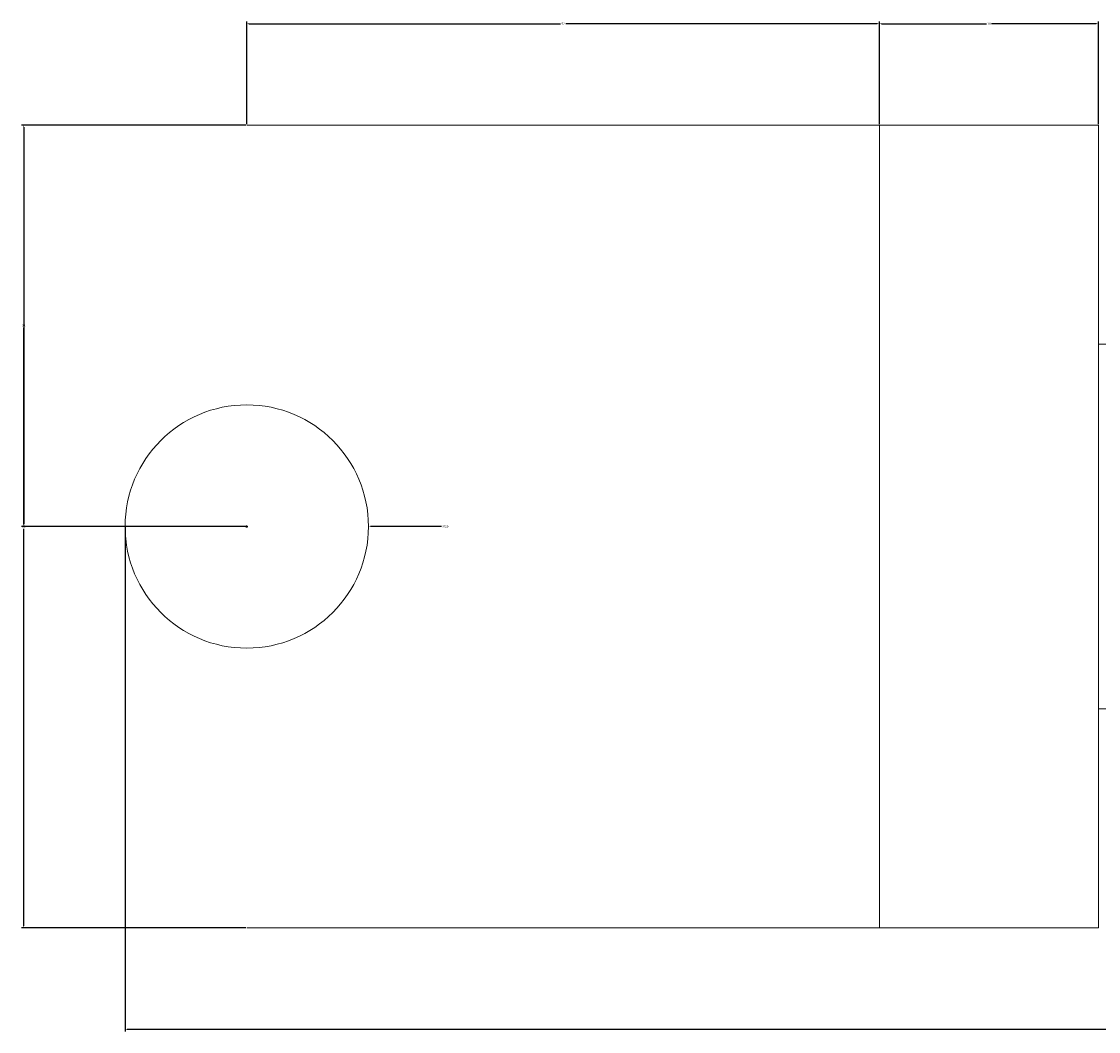
# Model space of a CAD drawing. Units: millimetres. Extents: x 2117 to 2298, y 1328 to 1411.
# Tile 1 of 3: x 2117 to 2205, y 1328 to 1411. Entities that reach past the tile are written whole.
import ezdxf

# ---------------------------------------------------------------- set-up
doc = ezdxf.new("R2010")
doc.units = ezdxf.units.MM
doc.layers.add('M-CONS', color=8, linetype='Continuous', lineweight=18)
doc.layers.add('M-DIMS', color=2, linetype='Continuous', lineweight=18)
doc.styles.get("Standard").update_dxf_attribs({"font": 'arial.ttf'})
doc.dimstyles.get("Standard").update_dxf_attribs({"dimtxt": 0.18, "dimasz": 0.18, "dimexe": 0.18, "dimexo": 0.0625, "dimgap": 0.09, "dimtad": 0, "dimtih": 1, "dimtoh": 1, "dimdec": 4, "dimzin": 0, "dimdsep": 46, "dimtxsty": 'Standard', "dimcen": 0.09, "dimadec": 0, "dimazin": 0, "dimtfac": 1, "dimtdec": 4, "dimtofl": 0, "dimtmove": 0, "dimatfit": 3, "dimfxl": 1, "dimtolj": 1, "dimtzin": 0, "dimarcsym": 0})

# ---------------------------------------------------------------- blocks, each defined once
blk = doc.blocks.new('*D3')
at = {"layer": 'Defpoints', "color": 0, "transparency": 16777216}
for p in [(2117.086, 1402.783), (2135.416, 1402.783), (2135.416, 1369.783)]:
    blk.add_point(p, dxfattribs=at)
at = {"layer": 'M-DIMS', "color": 0, "lineweight": -2, "transparency": 16777216}
for p, q in [((2135.354, 1402.783), (2116.906, 1402.783)), ((2117.086, 1402.603), (2117.086, 1386.465)), ((2117.086, 1369.963), (2117.086, 1386.101)), ((2135.354, 1369.783), (2116.906, 1369.783))]:
    blk.add_line(p, q, dxfattribs=at)
at = {"layer": 'M-DIMS', "color": 0, "transparency": 16777216}
for points in [[(2117.056, 1402.603), (2117.116, 1402.603), (2117.086, 1402.783)], [(2117.056, 1369.963), (2117.116, 1369.963), (2117.086, 1369.783)]]:
    blk.add_solid(points, dxfattribs=at)
at = {"layer": 'M-DIMS', "color": 0, "transparency": 16777216, "insert": (2117.086, 1386.283), "char_height": 0.18, "attachment_point": 5}
blk.add_mtext('\\A1;33', dxfattribs=at)
blk = doc.blocks.new('*D4')
at = {"layer": 'Defpoints', "color": 0, "transparency": 16777216}
for p in [(2117.086, 1402.783), (2135.416, 1402.783), (2135.416, 1336.783)]:
    blk.add_point(p, dxfattribs=at)
at = {"layer": 'M-DIMS', "color": 0, "lineweight": -2, "transparency": 16777216}
for p, q in [((2135.354, 1402.783), (2116.906, 1402.783)), ((2117.086, 1402.603), (2117.086, 1369.965)), ((2117.086, 1336.963), (2117.086, 1369.601)), ((2135.354, 1336.783), (2116.906, 1336.783))]:
    blk.add_line(p, q, dxfattribs=at)
at = {"layer": 'M-DIMS', "color": 0, "transparency": 16777216}
for points in [[(2117.056, 1402.603), (2117.116, 1402.603), (2117.086, 1402.783)], [(2117.056, 1336.963), (2117.116, 1336.963), (2117.086, 1336.783)]]:
    blk.add_solid(points, dxfattribs=at)
at = {"layer": 'M-DIMS', "color": 0, "transparency": 16777216, "insert": (2117.086, 1369.783), "char_height": 0.18, "attachment_point": 5}
blk.add_mtext('\\A1;66', dxfattribs=at)
blk = doc.blocks.new('*D5')
at = {"layer": 'Defpoints', "color": 0, "transparency": 16777216}
for p in [(2187.416, 1411.113), (2135.416, 1402.783), (2187.416, 1402.783)]:
    blk.add_point(p, dxfattribs=at)
at = {"layer": 'M-DIMS', "color": 0, "lineweight": -2, "transparency": 16777216}
for p, q in [((2135.416, 1402.845), (2135.416, 1411.293)), ((2135.596, 1411.113), (2161.198, 1411.113)), ((2187.236, 1411.113), (2161.634, 1411.113)), ((2187.416, 1402.845), (2187.416, 1411.293))]:
    blk.add_line(p, q, dxfattribs=at)
at = {"layer": 'M-DIMS', "color": 0, "transparency": 16777216}
for points in [[(2135.596, 1411.143), (2135.596, 1411.083), (2135.416, 1411.113)], [(2187.236, 1411.143), (2187.236, 1411.083), (2187.416, 1411.113)]]:
    blk.add_solid(points, dxfattribs=at)
at = {"layer": 'M-DIMS', "color": 0, "transparency": 16777216, "insert": (2161.416, 1411.113), "char_height": 0.18, "attachment_point": 5}
blk.add_mtext('\\A1;52', dxfattribs=at)
blk = doc.blocks.new('*D6')
at = {"layer": 'Defpoints', "color": 0, "transparency": 16777216}
for p in [(2205.416, 1411.113), (2187.416, 1402.783), (2205.416, 1402.783)]:
    blk.add_point(p, dxfattribs=at)
at = {"layer": 'M-DIMS', "color": 0, "lineweight": -2, "transparency": 16777216}
for p, q in [((2187.416, 1402.845), (2187.416, 1411.293)), ((2187.596, 1411.113), (2196.205, 1411.113)), ((2205.236, 1411.113), (2196.627, 1411.113)), ((2205.416, 1402.845), (2205.416, 1411.293))]:
    blk.add_line(p, q, dxfattribs=at)
at = {"layer": 'M-DIMS', "color": 0, "transparency": 16777216}
for points in [[(2187.596, 1411.143), (2187.596, 1411.083), (2187.416, 1411.113)], [(2205.236, 1411.143), (2205.236, 1411.083), (2205.416, 1411.113)]]:
    blk.add_solid(points, dxfattribs=at)
at = {"layer": 'M-DIMS', "color": 0, "transparency": 16777216, "insert": (2196.416, 1411.113), "char_height": 0.18, "attachment_point": 5}
blk.add_mtext('\\A1;18', dxfattribs=at)
blk = doc.blocks.new('*D12')
at = {"layer": 'Defpoints', "color": 0, "transparency": 16777216}
for p in [(2125.416, 1369.783), (2289.916, 1354.783), (2289.916, 1328.453)]:
    blk.add_point(p, dxfattribs=at)
at = {"layer": 'M-DIMS', "color": 0, "lineweight": -2, "transparency": 16777216}
for p, q in [((2125.416, 1369.72), (2125.416, 1328.273)), ((2289.916, 1354.72), (2289.916, 1328.273)), ((2125.596, 1328.453), (2207.28, 1328.453)), ((2289.736, 1328.453), (2208.052, 1328.453))]:
    blk.add_line(p, q, dxfattribs=at)
at = {"layer": 'M-DIMS', "color": 0, "transparency": 16777216}
for points in [[(2125.596, 1328.483), (2125.596, 1328.423), (2125.416, 1328.453)], [(2289.736, 1328.483), (2289.736, 1328.423), (2289.916, 1328.453)]]:
    blk.add_solid(points, dxfattribs=at)
at = {"layer": 'M-DIMS', "color": 0, "transparency": 16777216, "insert": (2207.666, 1328.453), "char_height": 0.18, "attachment_point": 5}
blk.add_mtext('\\A1;164.5', dxfattribs=at)
blk = doc.blocks.new('*D13')
at = {"layer": 'Defpoints', "color": 0, "transparency": 16777216}
for p in [(2125.416, 1369.783), (2145.416, 1369.783)]:
    blk.add_point(p, dxfattribs=at)
at = {"layer": 'M-DIMS', "color": 0, "lineweight": -2, "transparency": 16777216}
for p, q in [((2135.326, 1369.783), (2135.506, 1369.783)), ((2135.416, 1369.693), (2135.416, 1369.873)), ((2151.416, 1369.783), (2145.596, 1369.783))]:
    blk.add_line(p, q, dxfattribs=at)
at = {"layer": 'M-DIMS', "color": 0, "transparency": 16777216}
blk.add_solid([(2145.596, 1369.813), (2145.596, 1369.753), (2145.416, 1369.783)], dxfattribs=at)
at = {"layer": 'M-DIMS', "color": 0, "transparency": 16777216, "insert": (2151.733, 1369.783), "char_height": 0.18, "attachment_point": 5}
blk.add_mtext('\\A1;∅20', dxfattribs=at)

msp = doc.modelspace()

# ---------------------------------------------------------------- linework, layer by layer
at = {"layer": 'M-CONS'}
for points in [[(2135.416, 1402.783), (2205.416, 1402.783), (2187.416, 1402.783), (2187.416, 1336.783)], [(2205.416, 1402.783), (2205.416, 1336.783), (2135.416, 1336.783)], [(2205.416, 1369.783), (2205.416, 1384.783), (2277.416, 1384.783), (2277.416, 1354.783), (2205.416, 1354.783)]]:
    msp.add_lwpolyline(points, dxfattribs=at)
msp.add_circle((2135.416, 1369.783), 10, dxfattribs=at)

# ---------------------------------------------------------------- dimensions: what is measured, and where the dimension line sits
at = {"layer": 'M-DIMS'}
for base, p1, p2, override, picture, middle in [((2187.416, 1411.113), (2135.416, 1402.783), (2187.416, 1402.783), {"dimdec": 0, "dimlfac": 1, "dimrnd": 0, "dimzin": 0, "dimdsep": 46, "dimlunit": 2}, '*D5', (2161.416, 1411.113)), ((2205.416, 1411.113), (2187.416, 1402.783), (2205.416, 1402.783), {"dimdec": 0, "dimlfac": 1, "dimrnd": 0, "dimzin": 0, "dimdsep": 46, "dimlunit": 2}, '*D6', (2196.416, 1411.113)), ((2289.916, 1328.453), (2125.416, 1369.783), (2289.916, 1354.783), {"dimdec": 1, "dimlfac": 1, "dimrnd": 0, "dimzin": 0, "dimdsep": 46, "dimlunit": 2}, '*D12', (2207.666, 1328.453))]:
    dim = msp.add_linear_dim(base=base, p1=p1, p2=p2, dimstyle='Standard', override=override, dxfattribs=at)
    dim.commit()
    dim.dimension.update_dxf_attribs({"geometry": picture, "text_midpoint": middle})
for p1, picture, middle in [((2135.416, 1369.783), '*D3', (2117.086, 1386.283)), ((2135.416, 1336.783), '*D4', (2117.086, 1369.783))]:
    dim = msp.add_linear_dim(base=(2117.086, 1402.783), p1=p1, p2=(2135.416, 1402.783), angle=90, dimstyle='Standard', override={"dimdec": 0, "dimlfac": 1, "dimrnd": 0, "dimzin": 0, "dimdsep": 46, "dimlunit": 2}, dxfattribs=at)
    dim.commit()
    dim.dimension.update_dxf_attribs({"geometry": picture, "text_midpoint": middle})
dim = msp.add_diameter_dim_2p(p1=(2125.416, 1369.783), p2=(2145.416, 1369.783), dimstyle='Standard', override={"dimdec": 0, "dimlfac": 1, "dimrnd": 0, "dimzin": 0, "dimdsep": 46, "dimlunit": 2}, dxfattribs=at)
dim.commit()
dim.dimension.update_dxf_attribs({"geometry": '*D13', "text_midpoint": (2151.416, 1369.783), "dimtype": 163})

doc.saveas('drawing.dxf')
